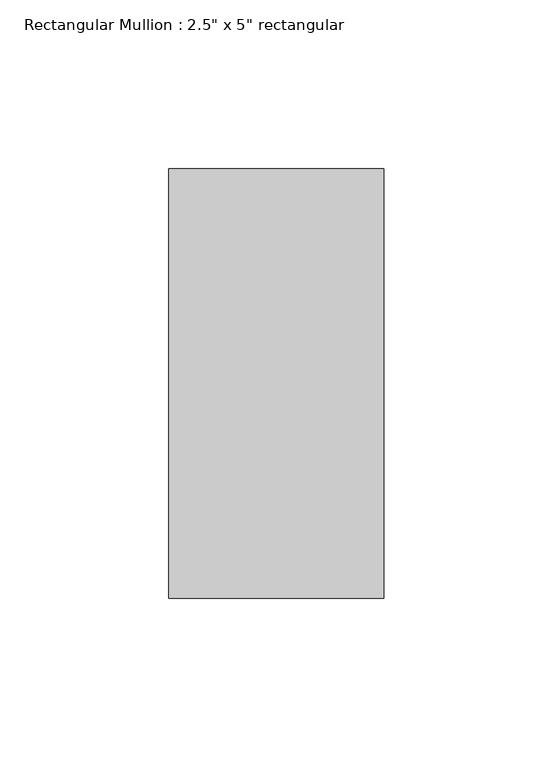
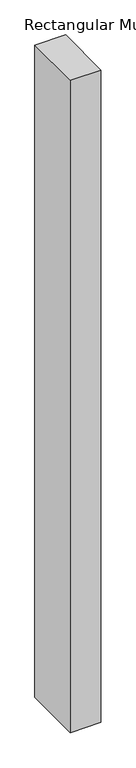
"""IFC4 building model written with IfcOpenShell, lengths in millimetres: member geometry."""

from ifc_helpers import new_model, si_unit, frame, origin, place, context, project, spatial, polyline, outline, extrude, source, transform, mapped, element, save


def member_c72ed4d9(model_context):
    return source(origin(), model_context, "Body", "SweptSolid", [
        extrude(outline(polyline([(31.75, 63.5), (31.75, -63.5), (-31.75, -63.5), (-31.75, 63.5), (31.75, 63.5)])), frame((0.0, 0.0, -1432.9498103), z_axis=(0.0, 0.0, 1.0), x_axis=(1.0, 0.0, 0.0)), (0.0, 0.0, 1.0), 1432.9498103),
    ])


if __name__ == "__main__":
    model = new_model("IFC4")
    model_context = context("Model", 3, world=origin())
    ifc_project = project(units=[si_unit("LENGTHUNIT", "METRE", prefix="MILLI")], contexts=[model_context])
    site = spatial("IfcSite", under=ifc_project)
    building = spatial("IfcBuilding", under=site)
    placement = place(None, origin())
    member_shape = member_c72ed4d9(model_context)
    element("IfcMember", 1, ObjectType="Rectangular Mullion : 2.5\" x 5\" rectangular", at=placement, inside=building, context=model_context, shape_type="MappedRepresentation", body=[
        mapped(member_shape, transform((0.0, 0.0, 0.0), x_axis=(1.0, 0.0, 0.0), y_axis=(0.0, 1.0, 0.0), z_axis=(0.0, 0.0, 1.0))),
    ])
    save(model, "model.ifc")

# Revit data of these elements
# Type "Rectangular Mullion : 2.5\" x 5\" rectangular"
#   built-in parameter 1007304 = 0.416667 (stored number, unit not read)
#   built-in parameter 1007301 = 0.104167 (stored number, unit not read)
#   built-in parameter 1007300 = 0.104167 (stored number, unit not read)
# Element 1 (IfcMember, "Rectangular Mullion : 2.5\" x 5\" rectangular")
#   Materials on its faces: "Aluminum"
# Materials
#   "Aluminum": class "Metal", colour RGB 247 247 247, transparency 0, Description = "Aluminum 6061", Cost = 0
